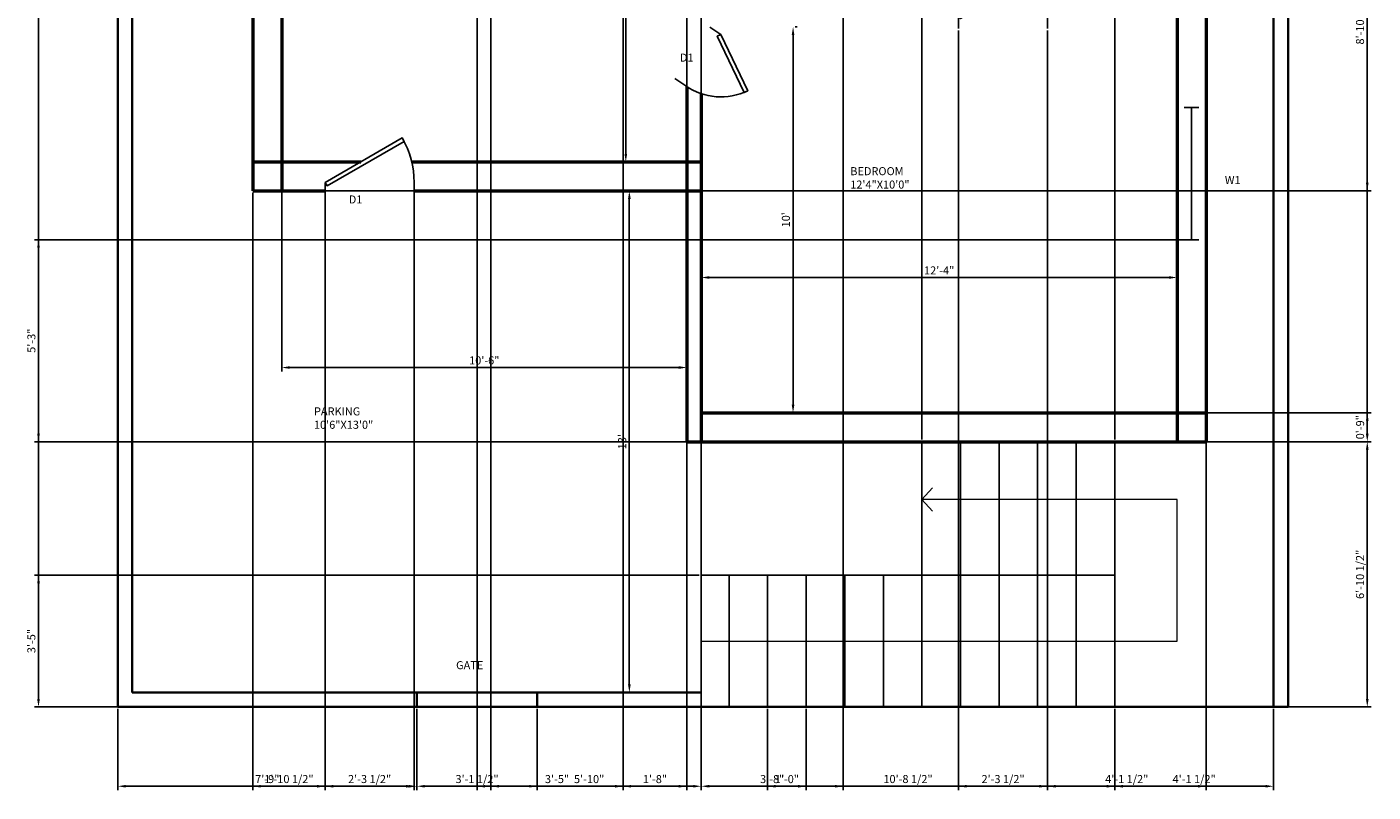
# Model space of a CAD drawing. Units: millimetres. Extents: x 2177 to 2598, y 1637 to 2185.
# Tile 1 of 2: x 2179 to 2598, y 1637 to 1875. Entities that reach past the tile are written whole.
import ezdxf

# ---------------------------------------------------------------- set-up
doc = ezdxf.new("R2010")
doc.units = ezdxf.units.MM
for name, color, linetype, lineweight in [('A-ANNO-DIMS', 150, 'Continuous', 18), ('A-ANNO-SYMB', 50, 'Continuous', 18), ('A-ANNO-TEXT', 40, 'Continuous', 18), ('A-AREA-IDEN', 40, 'Continuous', 25), ('A-WALL-SITE', 100, 'Continuous', 35), ('door', 130, 'Continuous', 25), ('steps', 50, 'Continuous', 25), ('walls', 100, 'Continuous', 50), ('windows', 10, 'Continuous', 25)]:
    doc.layers.add(name, color=color, linetype=linetype, lineweight=lineweight)
doc.styles.get("Standard").update_dxf_attribs({"font": 'arial.ttf'})
doc.dimstyles.new('ISO-25', dxfattribs={"dimtxt": 2.5, "dimasz": 2.5, "dimexe": 1.25, "dimexo": 0.625, "dimtad": 1, "dimlunit": 3, "dimtxsty": 'Standard', "dimcen": 2.5, "dimadec": 0, "dimazin": 0, "dimtfac": 1, "dimtmove": 0, "dimatfit": 3, "dimfxl": 1, "dimarcsym": 0})

# ---------------------------------------------------------------- blocks, each defined once
blk = doc.blocks.new('*U2')
for p, q in [((0, 0), (0, -6)), ((40, 0), (40, -6))]:
    blk.add_line(p, q)
blk.add_lwpolyline([(0, 0), (34.64, 20), (35.52, 18.48), (0.87, -1.52)], close=True)
blk.add_arc((0, 0), 40, 0, 30)
blk = doc.blocks.new('*U5')
for p, q in [((0, 0), (0, -6)), ((28, 0), (28, -6))]:
    blk.add_line(p, q)
blk.add_lwpolyline([(0, 0), (14, 24.25), (15.52, 23.37), (1.52, -0.88)], close=True)
blk.add_arc((0, 0), 28, 0, 60)
blk = doc.blocks.new('*U7')
for p, q in [((0, 4), (0, 0)), ((36, 4), (36, 0)), ((0, 2), (36, 2))]:
    blk.add_line(p, q)
blk = doc.blocks.new('*D15')
at = {"layer": 'A-ANNO-DIMS', "color": 0, "lineweight": -2, "transparency": 16777216}
for p, q in [((2344.56, 1989.02), (2366.75, 1989.02)), ((2365.5, 1835.52), (2365.5, 1986.52)), ((2344.56, 1833.02), (2366.75, 1833.02))]:
    blk.add_line(p, q, dxfattribs=at)
at = {"layer": 'A-ANNO-DIMS', "color": 0, "transparency": 16777216}
for points in [[(2365.08, 1986.52), (2365.91, 1986.52), (2365.5, 1989.02)], [(2365.08, 1835.52), (2365.91, 1835.52), (2365.5, 1833.02)]]:
    blk.add_solid(points, dxfattribs=at)
at = {"layer": 'Defpoints', "color": 0, "transparency": 16777216}
for p in [(2343.93, 1989.02), (2365.5, 1989.02), (2343.93, 1833.02)]:
    blk.add_point(p, dxfattribs=at)
at = {"layer": 'A-ANNO-DIMS', "color": 0, "transparency": 16777216, "insert": (2363.59, 1911.02), "char_height": 2.5, "attachment_point": 5, "rotation": 90}
blk.add_mtext("13'", dxfattribs=at)
blk = doc.blocks.new('*D16')
at = {"layer": 'A-ANNO-DIMS', "color": 0, "lineweight": -2, "transparency": 16777216}
for p, q in [((2344.93, 1824.02), (2367.84, 1824.02)), ((2366.59, 1821.52), (2366.59, 1670.52)), ((2344.93, 1668.02), (2367.84, 1668.02))]:
    blk.add_line(p, q, dxfattribs=at)
at = {"layer": 'A-ANNO-DIMS', "color": 0, "transparency": 16777216}
for points in [[(2366.18, 1821.52), (2367.01, 1821.52), (2366.59, 1824.02)], [(2366.18, 1670.52), (2367.01, 1670.52), (2366.59, 1668.02)]]:
    blk.add_solid(points, dxfattribs=at)
at = {"layer": 'Defpoints', "color": 0, "transparency": 16777216}
for p in [(2344.31, 1824.02), (2344.31, 1668.02), (2366.59, 1668.02)]:
    blk.add_point(p, dxfattribs=at)
at = {"layer": 'A-ANNO-DIMS', "color": 0, "transparency": 16777216, "insert": (2364.69, 1746.02), "char_height": 2.5, "attachment_point": 5, "rotation": 90}
blk.add_mtext("13'", dxfattribs=at)
blk = doc.blocks.new('*D17')
at = {"layer": 'A-ANNO-DIMS', "color": 0, "lineweight": -2, "transparency": 16777216}
for p, q in [((2258.47, 1832.4), (2258.47, 1767.82)), ((2384.47, 1832.4), (2384.47, 1767.82)), ((2260.97, 1769.07), (2381.97, 1769.07))]:
    blk.add_line(p, q, dxfattribs=at)
at = {"layer": 'A-ANNO-DIMS', "color": 0, "transparency": 16777216}
for points in [[(2260.97, 1769.49), (2260.97, 1768.66), (2258.47, 1769.07)], [(2381.97, 1769.49), (2381.97, 1768.66), (2384.47, 1769.07)]]:
    blk.add_solid(points, dxfattribs=at)
at = {"layer": 'Defpoints', "color": 0, "transparency": 16777216}
for p in [(2258.47, 1833.02), (2384.47, 1833.02), (2384.47, 1769.07)]:
    blk.add_point(p, dxfattribs=at)
at = {"layer": 'A-ANNO-DIMS', "color": 0, "transparency": 16777216, "insert": (2321.47, 1770.97), "char_height": 2.5, "attachment_point": 5}
blk.add_mtext('10\'-6"', dxfattribs=at)
blk = doc.blocks.new('*D18')
at = {"layer": 'A-ANNO-DIMS', "color": 0, "lineweight": -2, "transparency": 16777216}
for p, q in [((2417.52, 1757.52), (2417.52, 1872.52)), ((2418.14, 1875.02), (2418.77, 1875.02)), ((2418.14, 1755.02), (2418.77, 1755.02))]:
    blk.add_line(p, q, dxfattribs=at)
at = {"layer": 'A-ANNO-DIMS', "color": 0, "transparency": 16777216}
for points in [[(2417.1, 1872.52), (2417.93, 1872.52), (2417.52, 1875.02)], [(2417.1, 1757.52), (2417.93, 1757.52), (2417.52, 1755.02)]]:
    blk.add_solid(points, dxfattribs=at)
at = {"layer": 'Defpoints', "color": 0, "transparency": 16777216}
for p in [(2417.52, 1875.02), (2417.52, 1875.02), (2417.52, 1755.02)]:
    blk.add_point(p, dxfattribs=at)
at = {"layer": 'A-ANNO-DIMS', "color": 0, "transparency": 16777216, "insert": (2415.61, 1815.02), "char_height": 2.5, "attachment_point": 5, "rotation": 90}
blk.add_mtext("10'", dxfattribs=at)
blk = doc.blocks.new('*D19')
at = {"layer": 'A-ANNO-DIMS', "color": 0, "lineweight": -2, "transparency": 16777216}
for p, q in [((2388.97, 1812.3), (2388.97, 1795.82)), ((2536.97, 1812.3), (2536.97, 1795.82)), ((2391.47, 1797.07), (2534.47, 1797.07))]:
    blk.add_line(p, q, dxfattribs=at)
at = {"layer": 'A-ANNO-DIMS', "color": 0, "transparency": 16777216}
for points in [[(2391.47, 1797.49), (2391.47, 1796.66), (2388.97, 1797.07)], [(2534.47, 1797.49), (2534.47, 1796.66), (2536.97, 1797.07)]]:
    blk.add_solid(points, dxfattribs=at)
at = {"layer": 'Defpoints', "color": 0, "transparency": 16777216}
for p in [(2388.97, 1812.93), (2536.97, 1812.93), (2536.97, 1797.07)]:
    blk.add_point(p, dxfattribs=at)
at = {"layer": 'A-ANNO-DIMS', "color": 0, "transparency": 16777216, "insert": (2462.97, 1798.95), "char_height": 2.5, "attachment_point": 5}
blk.add_mtext('12\'-4"', dxfattribs=at)
blk = doc.blocks.new('*D25')
at = {"layer": 'A-ANNO-DIMS', "color": 0, "lineweight": -2, "transparency": 16777216}
for p, q in [((2206.84, 2154.52), (2181.57, 2154.52)), ((2182.82, 1666.02), (2182.82, 2152.02)), ((2206.84, 1663.52), (2181.57, 1663.52))]:
    blk.add_line(p, q, dxfattribs=at)
at = {"layer": 'A-ANNO-DIMS', "color": 0, "transparency": 16777216}
for points in [[(2182.4, 2152.02), (2183.24, 2152.02), (2182.82, 2154.52)], [(2182.4, 1666.02), (2183.24, 1666.02), (2182.82, 1663.52)]]:
    blk.add_solid(points, dxfattribs=at)
at = {"layer": 'Defpoints', "color": 0, "transparency": 16777216}
for p in [(2182.82, 2154.52), (2207.47, 2154.52), (2207.47, 1663.52)]:
    blk.add_point(p, dxfattribs=at)
at = {"layer": 'A-ANNO-DIMS', "color": 0, "transparency": 16777216, "insert": (2180.92, 1909.02), "char_height": 2.5, "attachment_point": 5, "rotation": 90}
blk.add_mtext('40\'-11"', dxfattribs=at)
blk = doc.blocks.new('*D27')
at = {"layer": 'A-ANNO-DIMS', "color": 0, "lineweight": -2, "transparency": 16777216}
for p, q in [((2546.59, 2122.52), (2597.37, 2122.52)), ((2596.12, 2120.02), (2596.12, 1748.52)), ((2546.59, 1746.02), (2597.37, 1746.02))]:
    blk.add_line(p, q, dxfattribs=at)
at = {"layer": 'A-ANNO-DIMS', "color": 0, "transparency": 16777216}
for points in [[(2595.7, 2120.02), (2596.54, 2120.02), (2596.12, 2122.52)], [(2595.7, 1748.52), (2596.54, 1748.52), (2596.12, 1746.02)]]:
    blk.add_solid(points, dxfattribs=at)
at = {"layer": 'Defpoints', "color": 0, "transparency": 16777216}
for p in [(2545.97, 2122.52), (2545.97, 1746.02), (2596.12, 1746.02)]:
    blk.add_point(p, dxfattribs=at)
at = {"layer": 'A-ANNO-DIMS', "color": 0, "transparency": 16777216, "insert": (2594.2, 1934.27), "char_height": 2.5, "attachment_point": 5, "rotation": 90}
blk.add_mtext('31\'-4 1/2"', dxfattribs=at)
blk = doc.blocks.new('*D28')
at = {"layer": 'A-ANNO-DIMS', "color": 0, "lineweight": -2, "transparency": 16777216}
for p, q in [((2546.59, 1755.02), (2597.37, 1755.02)), ((2596.12, 1752.52), (2596.12, 1748.52)), ((2546.59, 1746.02), (2597.37, 1746.02))]:
    blk.add_line(p, q, dxfattribs=at)
at = {"layer": 'A-ANNO-DIMS', "color": 0, "transparency": 16777216}
for points in [[(2595.7, 1752.52), (2596.54, 1752.52), (2596.12, 1755.02)], [(2595.7, 1748.52), (2596.54, 1748.52), (2596.12, 1746.02)]]:
    blk.add_solid(points, dxfattribs=at)
at = {"layer": 'Defpoints', "color": 0, "transparency": 16777216}
for p in [(2545.97, 1755.02), (2545.97, 1746.02), (2596.12, 1746.02)]:
    blk.add_point(p, dxfattribs=at)
at = {"layer": 'A-ANNO-DIMS', "color": 0, "transparency": 16777216, "insert": (2594.22, 1750.52), "char_height": 2.5, "attachment_point": 5, "rotation": 90}
blk.add_mtext('0\'-9"', dxfattribs=at)
blk = doc.blocks.new('*D30')
at = {"layer": 'A-ANNO-DIMS', "color": 0, "lineweight": -2, "transparency": 16777216}
for p, q in [((2300.47, 1662.9), (2300.47, 1637.62)), ((2337.97, 1662.9), (2337.97, 1637.62)), ((2302.97, 1638.87), (2335.47, 1638.87))]:
    blk.add_line(p, q, dxfattribs=at)
at = {"layer": 'A-ANNO-DIMS', "color": 0, "transparency": 16777216}
for points in [[(2302.97, 1639.29), (2302.97, 1638.46), (2300.47, 1638.87)], [(2335.47, 1639.29), (2335.47, 1638.46), (2337.97, 1638.87)]]:
    blk.add_solid(points, dxfattribs=at)
at = {"layer": 'Defpoints', "color": 0, "transparency": 16777216}
for p in [(2300.47, 1663.52), (2337.97, 1663.52), (2337.97, 1638.87)]:
    blk.add_point(p, dxfattribs=at)
at = {"layer": 'A-ANNO-DIMS', "color": 0, "transparency": 16777216, "insert": (2319.22, 1640.79), "char_height": 2.5, "attachment_point": 5}
blk.add_mtext('3\'-1 1/2"', dxfattribs=at)
blk = doc.blocks.new('*D31')
at = {"layer": 'A-ANNO-DIMS', "color": 0, "lineweight": -2, "transparency": 16777216}
for p, q in [((2207.47, 1662.9), (2207.47, 1637.62)), ((2300.47, 1662.9), (2300.47, 1637.62)), ((2209.97, 1638.87), (2297.97, 1638.87))]:
    blk.add_line(p, q, dxfattribs=at)
at = {"layer": 'A-ANNO-DIMS', "color": 0, "transparency": 16777216}
for points in [[(2209.97, 1639.29), (2209.97, 1638.46), (2207.47, 1638.87)], [(2297.97, 1639.29), (2297.97, 1638.46), (2300.47, 1638.87)]]:
    blk.add_solid(points, dxfattribs=at)
at = {"layer": 'Defpoints', "color": 0, "transparency": 16777216}
for p in [(2207.47, 1663.52), (2300.47, 1663.52), (2300.47, 1638.87)]:
    blk.add_point(p, dxfattribs=at)
at = {"layer": 'A-ANNO-DIMS', "color": 0, "transparency": 16777216, "insert": (2253.97, 1640.77), "char_height": 2.5, "attachment_point": 5}
blk.add_mtext('7\'-9"', dxfattribs=at)
blk = doc.blocks.new('*D32')
at = {"layer": 'A-ANNO-DIMS', "color": 0, "lineweight": -2, "transparency": 16777216}
for p, q in [((2271.98, 1823.4), (2271.98, 1637.62)), ((2299.64, 1823.4), (2299.64, 1637.62)), ((2274.48, 1638.87), (2297.14, 1638.87))]:
    blk.add_line(p, q, dxfattribs=at)
at = {"layer": 'A-ANNO-DIMS', "color": 0, "transparency": 16777216}
for points in [[(2274.48, 1639.29), (2274.48, 1638.46), (2271.98, 1638.87)], [(2297.14, 1639.29), (2297.14, 1638.46), (2299.64, 1638.87)]]:
    blk.add_solid(points, dxfattribs=at)
at = {"layer": 'Defpoints', "color": 0, "transparency": 16777216}
for p in [(2271.98, 1824.02), (2299.64, 1824.02), (2299.64, 1638.87)]:
    blk.add_point(p, dxfattribs=at)
at = {"layer": 'A-ANNO-DIMS', "color": 0, "transparency": 16777216, "insert": (2285.81, 1640.79), "char_height": 2.5, "attachment_point": 5}
blk.add_mtext('2\'-3 1/2"', dxfattribs=at)
blk = doc.blocks.new('*D33')
at = {"layer": 'A-ANNO-DIMS', "color": 0, "lineweight": -2, "transparency": 16777216}
for p, q in [((2323.55, 2116.57), (2323.55, 1637.62)), ((2364.65, 2116.57), (2364.65, 1637.62)), ((2326.05, 1638.87), (2362.15, 1638.87))]:
    blk.add_line(p, q, dxfattribs=at)
at = {"layer": 'A-ANNO-DIMS', "color": 0, "transparency": 16777216}
for points in [[(2326.05, 1639.29), (2326.05, 1638.46), (2323.55, 1638.87)], [(2362.15, 1639.29), (2362.15, 1638.46), (2364.65, 1638.87)]]:
    blk.add_solid(points, dxfattribs=at)
at = {"layer": 'Defpoints', "color": 0, "transparency": 16777216}
for p in [(2323.55, 2117.19), (2364.65, 2117.19), (2364.65, 1638.87)]:
    blk.add_point(p, dxfattribs=at)
at = {"layer": 'A-ANNO-DIMS', "color": 0, "transparency": 16777216, "insert": (2344.1, 1640.78), "char_height": 2.5, "attachment_point": 5}
blk.add_mtext('3\'-5"', dxfattribs=at)
blk = doc.blocks.new('*D35')
at = {"layer": 'A-ANNO-DIMS', "color": 0, "lineweight": -2, "transparency": 16777216}
for p, q in [((2457.6, 1746.65), (2457.6, 2180.42)), ((2460.1, 2179.17), (2515.1, 2179.17)), ((2517.6, 1746.65), (2517.6, 2180.42))]:
    blk.add_line(p, q, dxfattribs=at)
at = {"layer": 'A-ANNO-DIMS', "color": 0, "transparency": 16777216}
for points in [[(2460.1, 2179.59), (2460.1, 2178.76), (2457.6, 2179.17)], [(2515.1, 2179.59), (2515.1, 2178.76), (2517.6, 2179.17)]]:
    blk.add_solid(points, dxfattribs=at)
at = {"layer": 'Defpoints', "color": 0, "transparency": 16777216}
for p in [(2517.6, 2179.17), (2457.6, 1746.02), (2517.6, 1746.02)]:
    blk.add_point(p, dxfattribs=at)
at = {"layer": 'A-ANNO-DIMS', "color": 0, "transparency": 16777216, "insert": (2487.6, 2181.07), "char_height": 2.5, "attachment_point": 5}
blk.add_mtext('5\'-0"', dxfattribs=at)
blk = doc.blocks.new('*D36')
at = {"layer": 'A-ANNO-DIMS', "color": 0, "lineweight": -2, "transparency": 16777216}
for p, q in [((2409.6, 1662.9), (2409.6, 1637.62)), ((2421.6, 1662.9), (2421.6, 1637.62)), ((2412.1, 1638.87), (2419.1, 1638.87))]:
    blk.add_line(p, q, dxfattribs=at)
at = {"layer": 'A-ANNO-DIMS', "color": 0, "transparency": 16777216}
for points in [[(2412.1, 1639.29), (2412.1, 1638.46), (2409.6, 1638.87)], [(2419.1, 1639.29), (2419.1, 1638.46), (2421.6, 1638.87)]]:
    blk.add_solid(points, dxfattribs=at)
at = {"layer": 'Defpoints', "color": 0, "transparency": 16777216}
for p in [(2409.6, 1663.52), (2421.6, 1663.52), (2421.6, 1638.87)]:
    blk.add_point(p, dxfattribs=at)
at = {"layer": 'A-ANNO-DIMS', "color": 0, "transparency": 16777216, "insert": (2415.6, 1640.77), "char_height": 2.5, "attachment_point": 5}
blk.add_mtext('1\'-0"', dxfattribs=at)
blk = doc.blocks.new('*D37')
at = {"layer": 'A-ANNO-DIMS', "color": 0, "lineweight": -2, "transparency": 16777216}
for p, q in [((2388.34, 1704.52), (2181.57, 1704.52)), ((2182.82, 1666.02), (2182.82, 1702.02)), ((2388.34, 1663.52), (2181.57, 1663.52))]:
    blk.add_line(p, q, dxfattribs=at)
at = {"layer": 'A-ANNO-DIMS', "color": 0, "transparency": 16777216}
for points in [[(2182.4, 1702.02), (2183.24, 1702.02), (2182.82, 1704.52)], [(2182.4, 1666.02), (2183.24, 1666.02), (2182.82, 1663.52)]]:
    blk.add_solid(points, dxfattribs=at)
at = {"layer": 'Defpoints', "color": 0, "transparency": 16777216}
for p in [(2182.82, 1704.52), (2388.97, 1704.52), (2388.97, 1663.52)]:
    blk.add_point(p, dxfattribs=at)
at = {"layer": 'A-ANNO-DIMS', "color": 0, "transparency": 16777216, "insert": (2180.92, 1684.02), "char_height": 2.5, "attachment_point": 5, "rotation": 90}
blk.add_mtext('3\'-5"', dxfattribs=at)
blk = doc.blocks.new('*D38')
at = {"layer": 'A-ANNO-DIMS', "color": 0, "lineweight": -2, "transparency": 16777216}
for p, q in [((2388.97, 1662.9), (2388.97, 1637.62)), ((2517.6, 1662.9), (2517.6, 1637.62)), ((2391.47, 1638.87), (2515.1, 1638.87))]:
    blk.add_line(p, q, dxfattribs=at)
at = {"layer": 'A-ANNO-DIMS', "color": 0, "transparency": 16777216}
for points in [[(2391.47, 1639.29), (2391.47, 1638.46), (2388.97, 1638.87)], [(2515.1, 1639.29), (2515.1, 1638.46), (2517.6, 1638.87)]]:
    blk.add_solid(points, dxfattribs=at)
at = {"layer": 'Defpoints', "color": 0, "transparency": 16777216}
for p in [(2388.97, 1663.52), (2517.6, 1663.52), (2517.6, 1638.87)]:
    blk.add_point(p, dxfattribs=at)
at = {"layer": 'A-ANNO-DIMS', "color": 0, "transparency": 16777216, "insert": (2453.28, 1640.79), "char_height": 2.5, "attachment_point": 5}
blk.add_mtext('10\'-8 1/2"', dxfattribs=at)
blk = doc.blocks.new('*D39')
at = {"layer": 'A-ANNO-DIMS', "color": 0, "lineweight": -2, "transparency": 16777216}
for p, q in [((2517.6, 1662.9), (2517.6, 1637.62)), ((2566.97, 1662.9), (2566.97, 1637.62)), ((2520.1, 1638.87), (2564.47, 1638.87))]:
    blk.add_line(p, q, dxfattribs=at)
at = {"layer": 'A-ANNO-DIMS', "color": 0, "transparency": 16777216}
for points in [[(2520.1, 1639.29), (2520.1, 1638.46), (2517.6, 1638.87)], [(2564.47, 1639.29), (2564.47, 1638.46), (2566.97, 1638.87)]]:
    blk.add_solid(points, dxfattribs=at)
at = {"layer": 'Defpoints', "color": 0, "transparency": 16777216}
for p in [(2517.6, 1663.52), (2566.97, 1663.52), (2566.97, 1638.87)]:
    blk.add_point(p, dxfattribs=at)
at = {"layer": 'A-ANNO-DIMS', "color": 0, "transparency": 16777216, "insert": (2542.28, 1640.79), "char_height": 2.5, "attachment_point": 5}
blk.add_mtext('4\'-1 1/2"', dxfattribs=at)
blk = doc.blocks.new('*D40')
at = {"layer": 'A-ANNO-DIMS', "color": 0, "lineweight": -2, "transparency": 16777216}
for p, q in [((2469.01, 1873.88), (2469.01, 1637.62)), ((2496.67, 1873.88), (2496.67, 1637.62)), ((2471.51, 1638.87), (2494.17, 1638.87))]:
    blk.add_line(p, q, dxfattribs=at)
at = {"layer": 'A-ANNO-DIMS', "color": 0, "transparency": 16777216}
for points in [[(2471.51, 1639.29), (2471.51, 1638.46), (2469.01, 1638.87)], [(2494.17, 1639.29), (2494.17, 1638.46), (2496.67, 1638.87)]]:
    blk.add_solid(points, dxfattribs=at)
at = {"layer": 'Defpoints', "color": 0, "transparency": 16777216}
for p in [(2469.01, 1874.51), (2496.67, 1874.51), (2496.67, 1638.87)]:
    blk.add_point(p, dxfattribs=at)
at = {"layer": 'A-ANNO-DIMS', "color": 0, "transparency": 16777216, "insert": (2482.84, 1640.79), "char_height": 2.5, "attachment_point": 5}
blk.add_mtext('2\'-3 1/2"', dxfattribs=at)
blk = doc.blocks.new('*D41')
at = {"layer": 'A-ANNO-DIMS', "color": 0, "lineweight": -2, "transparency": 16777216}
for p, q in [((2249.47, 1823.4), (2249.47, 1637.62)), ((2271.98, 1823.4), (2271.98, 1637.62)), ((2251.97, 1638.87), (2269.48, 1638.87))]:
    blk.add_line(p, q, dxfattribs=at)
at = {"layer": 'A-ANNO-DIMS', "color": 0, "transparency": 16777216}
for points in [[(2251.97, 1639.29), (2251.97, 1638.46), (2249.47, 1638.87)], [(2269.48, 1639.29), (2269.48, 1638.46), (2271.98, 1638.87)]]:
    blk.add_solid(points, dxfattribs=at)
at = {"layer": 'Defpoints', "color": 0, "transparency": 16777216}
for p in [(2249.47, 1824.02), (2271.98, 1824.02), (2271.98, 1638.87)]:
    blk.add_point(p, dxfattribs=at)
at = {"layer": 'A-ANNO-DIMS', "color": 0, "transparency": 16777216, "insert": (2260.72, 1640.79), "char_height": 2.5, "attachment_point": 5}
blk.add_mtext('1\'-10 1/2"', dxfattribs=at)
blk = doc.blocks.new('*D43')
at = {"layer": 'A-ANNO-DIMS', "color": 0, "lineweight": -2, "transparency": 16777216}
for p, q in [((2545.97, 1878.9), (2545.97, 1637.62)), ((2496.67, 1873.88), (2496.67, 1637.62)), ((2499.17, 1638.87), (2543.47, 1638.87))]:
    blk.add_line(p, q, dxfattribs=at)
at = {"layer": 'A-ANNO-DIMS', "color": 0, "transparency": 16777216}
for points in [[(2499.17, 1639.29), (2499.17, 1638.46), (2496.67, 1638.87)], [(2543.47, 1639.29), (2543.47, 1638.46), (2545.97, 1638.87)]]:
    blk.add_solid(points, dxfattribs=at)
at = {"layer": 'Defpoints', "color": 0, "transparency": 16777216}
for p in [(2545.97, 1879.52), (2496.67, 1874.51), (2545.97, 1638.87)]:
    blk.add_point(p, dxfattribs=at)
at = {"layer": 'A-ANNO-DIMS', "color": 0, "transparency": 16777216, "insert": (2521.32, 1640.79), "char_height": 2.5, "attachment_point": 5}
blk.add_mtext('4\'-1 1/2"', dxfattribs=at)
blk = doc.blocks.new('*D45')
at = {"layer": 'A-ANNO-DIMS', "color": 0, "lineweight": -2, "transparency": 16777216}
for p, q in [((2518.22, 1746.02), (2597.37, 1746.02)), ((2596.12, 1666.02), (2596.12, 1743.52)), ((2518.22, 1663.52), (2597.37, 1663.52))]:
    blk.add_line(p, q, dxfattribs=at)
at = {"layer": 'A-ANNO-DIMS', "color": 0, "transparency": 16777216}
for points in [[(2595.7, 1743.52), (2596.54, 1743.52), (2596.12, 1746.02)], [(2595.7, 1666.02), (2596.54, 1666.02), (2596.12, 1663.52)]]:
    blk.add_solid(points, dxfattribs=at)
at = {"layer": 'Defpoints', "color": 0, "transparency": 16777216}
for p in [(2517.6, 1746.02), (2596.12, 1746.02), (2517.6, 1663.52)]:
    blk.add_point(p, dxfattribs=at)
at = {"layer": 'A-ANNO-DIMS', "color": 0, "transparency": 16777216, "insert": (2594.2, 1704.77), "char_height": 2.5, "attachment_point": 5, "rotation": 90}
blk.add_mtext('6\'-10 1/2"', dxfattribs=at)
blk = doc.blocks.new('*D47')
at = {"layer": 'A-ANNO-DIMS', "color": 0, "lineweight": -2, "transparency": 16777216}
for p, q in [((2319.22, 1988.4), (2319.22, 1637.62)), ((2388.97, 1988.4), (2388.97, 1637.62)), ((2321.72, 1638.87), (2386.47, 1638.87))]:
    blk.add_line(p, q, dxfattribs=at)
at = {"layer": 'A-ANNO-DIMS', "color": 0, "transparency": 16777216}
for points in [[(2321.72, 1639.29), (2321.72, 1638.46), (2319.22, 1638.87)], [(2386.47, 1639.29), (2386.47, 1638.46), (2388.97, 1638.87)]]:
    blk.add_solid(points, dxfattribs=at)
at = {"layer": 'Defpoints', "color": 0, "transparency": 16777216}
for p in [(2319.22, 1989.02), (2388.97, 1989.02), (2388.97, 1638.87)]:
    blk.add_point(p, dxfattribs=at)
at = {"layer": 'A-ANNO-DIMS', "color": 0, "transparency": 16777216, "insert": (2354.09, 1640.77), "char_height": 2.5, "attachment_point": 5}
blk.add_mtext('5\'-10"', dxfattribs=at)
blk = doc.blocks.new('*D48')
at = {"layer": 'A-ANNO-DIMS', "color": 0, "lineweight": -2, "transparency": 16777216}
for p, q in [((2388.97, 2121.9), (2388.97, 1637.62)), ((2433.07, 2116.49), (2433.07, 1637.62)), ((2391.47, 1638.87), (2430.57, 1638.87))]:
    blk.add_line(p, q, dxfattribs=at)
at = {"layer": 'A-ANNO-DIMS', "color": 0, "transparency": 16777216}
for points in [[(2391.47, 1639.29), (2391.47, 1638.46), (2388.97, 1638.87)], [(2430.57, 1639.29), (2430.57, 1638.46), (2433.07, 1638.87)]]:
    blk.add_solid(points, dxfattribs=at)
at = {"layer": 'Defpoints', "color": 0, "transparency": 16777216}
for p in [(2388.97, 2122.52), (2433.07, 2117.11), (2433.07, 1638.87)]:
    blk.add_point(p, dxfattribs=at)
at = {"layer": 'A-ANNO-DIMS', "color": 0, "transparency": 16777216, "insert": (2411.02, 1640.78), "char_height": 2.5, "attachment_point": 5}
blk.add_mtext('3\'-8"', dxfattribs=at)
blk = doc.blocks.new('*D50')
at = {"layer": 'A-ANNO-DIMS', "color": 0, "lineweight": -2, "transparency": 16777216}
for p, q in [((2254.73, 1930.31), (2597.37, 1930.31)), ((2596.12, 1826.52), (2596.12, 1927.81)), ((2259.09, 1824.02), (2597.37, 1824.02))]:
    blk.add_line(p, q, dxfattribs=at)
at = {"layer": 'A-ANNO-DIMS', "color": 0, "transparency": 16777216}
for points in [[(2595.7, 1927.81), (2596.54, 1927.81), (2596.12, 1930.31)], [(2595.7, 1826.52), (2596.54, 1826.52), (2596.12, 1824.02)]]:
    blk.add_solid(points, dxfattribs=at)
at = {"layer": 'Defpoints', "color": 0, "transparency": 16777216}
for p in [(2254.11, 1930.31), (2596.12, 1930.31), (2258.47, 1824.02)]:
    blk.add_point(p, dxfattribs=at)
at = {"layer": 'A-ANNO-DIMS', "color": 0, "transparency": 16777216, "insert": (2594.2, 1877.17), "char_height": 2.5, "attachment_point": 5, "rotation": 90}
blk.add_mtext('8\'-10 1/2"', dxfattribs=at)
blk = doc.blocks.new('*D52')
at = {"layer": 'A-ANNO-DIMS', "color": 0, "lineweight": -2, "transparency": 16777216}
for p, q in [((2540.85, 1808.81), (2181.57, 1808.81)), ((2182.82, 1806.31), (2182.82, 1748.52)), ((2536.34, 1746.02), (2181.57, 1746.02))]:
    blk.add_line(p, q, dxfattribs=at)
at = {"layer": 'A-ANNO-DIMS', "color": 0, "transparency": 16777216}
for points in [[(2182.4, 1806.31), (2183.24, 1806.31), (2182.82, 1808.81)], [(2182.4, 1748.52), (2183.24, 1748.52), (2182.82, 1746.02)]]:
    blk.add_solid(points, dxfattribs=at)
at = {"layer": 'Defpoints', "color": 0, "transparency": 16777216}
for p in [(2541.47, 1808.81), (2182.82, 1746.02), (2536.97, 1746.02)]:
    blk.add_point(p, dxfattribs=at)
at = {"layer": 'A-ANNO-DIMS', "color": 0, "transparency": 16777216, "insert": (2180.92, 1777.42), "char_height": 2.5, "attachment_point": 5, "rotation": 90}
blk.add_mtext('5\'-3"', dxfattribs=at)
blk = doc.blocks.new('*D53')
at = {"layer": 'A-ANNO-DIMS', "color": 0, "lineweight": -2, "transparency": 16777216}
for p, q in [((2384.47, 2121.9), (2384.47, 1637.62)), ((2364.65, 2116.57), (2364.65, 1637.62)), ((2367.15, 1638.87), (2381.97, 1638.87))]:
    blk.add_line(p, q, dxfattribs=at)
at = {"layer": 'A-ANNO-DIMS', "color": 0, "transparency": 16777216}
for points in [[(2367.15, 1639.29), (2367.15, 1638.46), (2364.65, 1638.87)], [(2381.97, 1639.29), (2381.97, 1638.46), (2384.47, 1638.87)]]:
    blk.add_solid(points, dxfattribs=at)
at = {"layer": 'Defpoints', "color": 0, "transparency": 16777216}
for p in [(2384.47, 2122.52), (2364.65, 2117.19), (2384.47, 1638.87)]:
    blk.add_point(p, dxfattribs=at)
at = {"layer": 'A-ANNO-DIMS', "color": 0, "transparency": 16777216, "insert": (2374.56, 1640.77), "char_height": 2.5, "attachment_point": 5}
blk.add_mtext('1\'-8"', dxfattribs=at)

msp = doc.modelspace()

# ---------------------------------------------------------------- linework, layer by layer
at = {"layer": 'A-ANNO-SYMB'}
for p, q in [((2457.598, 1728.042), (2460.872, 1731.701)), ((2536.97, 1728.042), (2457.598, 1728.042)), ((2457.598, 1728.042), (2457.598, 1728.042)), ((2457.598, 1728.042), (2460.872, 1724.383)), ((2536.97, 1684.023), (2536.97, 1728.042)), ((2388.97, 1684.023), (2536.97, 1684.023))]:
    msp.add_line(p, q, dxfattribs=at)
at = {"layer": 'A-WALL-SITE'}
for p, q in [((2207.47, 2154.523), (2207.47, 1663.523)), ((2211.97, 2154.523), (2211.97, 1668.023)), ((2566.97, 1663.523), (2566.97, 2154.523)), ((2571.47, 1663.523), (2571.47, 2154.523)), ((2211.97, 1668.023), (2388.97, 1668.023)), ((2300.47, 1668.023), (2300.47, 1663.523)), ((2300.47, 1663.523), (2300.47, 1668.023)), ((2300.47, 1668.023), (2300.47, 1668.023)), ((2337.97, 1668.023), (2337.97, 1663.523)), ((2207.47, 1663.523), (2505.598, 1663.523)), ((2505.598, 1663.523), (2571.47, 1663.523))]:
    msp.add_line(p, q, dxfattribs=at)
at = {"layer": 'steps'}
for p, q in [((2388.97, 1746.023), (2388.97, 1663.523)), ((2388.97, 1746.023), (2388.97, 1705.023)), ((2457.598, 1746.023), (2457.598, 1663.523)), ((2469.598, 1746.023), (2469.598, 1663.523)), ((2481.598, 1746.023), (2481.598, 1663.523)), ((2493.598, 1746.023), (2493.598, 1663.523)), ((2505.598, 1746.023), (2505.598, 1663.523)), ((2517.598, 1704.523), (2517.598, 1746.023)), ((2517.598, 1746.023), (2517.598, 1663.523)), ((2388.97, 1663.523), (2388.97, 1704.523)), ((2388.97, 1663.523), (2388.97, 1704.523)), ((2388.97, 1704.523), (2517.598, 1704.523)), ((2397.598, 1704.523), (2397.598, 1663.523)), ((2409.598, 1704.523), (2409.598, 1663.523)), ((2421.598, 1704.523), (2421.598, 1663.523)), ((2433.598, 1704.523), (2433.598, 1663.523)), ((2445.598, 1704.523), (2445.598, 1663.523)), ((2388.97, 1663.523), (2388.97, 1699.523))]:
    msp.add_line(p, q, dxfattribs=at)
at = {"layer": 'walls'}
for p, q in [((2536.97, 2122.523), (2536.97, 1746.023)), ((2545.97, 2122.523), (2545.97, 1746.023)), ((2258.47, 2068.811), (2258.47, 1824.023)), ((2249.47, 2068.167), (2249.47, 1824.023)), ((2384.47, 1856.396), (2384.47, 1824.023)), ((2384.47, 1854.228), (2384.47, 1746.023)), ((2388.97, 1854.228), (2388.97, 1746.023)), ((2249.47, 1833.023), (2283.05, 1833.023)), ((2298.896, 1833.023), (2388.97, 1833.023)), ((2249.47, 1824.023), (2271.978, 1824.023)), ((2299.644, 1824.023), (2388.97, 1824.023)), ((2388.97, 1755.023), (2545.97, 1755.023)), ((2384.47, 1746.023), (2545.97, 1746.023))]:
    msp.add_line(p, q, dxfattribs=at)

# ---------------------------------------------------------------- block references
at = {"layer": 'door', "xscale": 0.6916711511996688, "yscale": 0.6916711511996688, "zscale": 0.6916711511996688}
for p in [(2469.006, 1878.656), (2271.978, 1826.63)]:
    msp.add_blockref('*U2', p, dxfattribs=at)
at = {"layer": 'door', "xscale": 0.6916711511996688, "yscale": 0.6916711511996688, "zscale": 0.6916711511996688, "rotation": 235.6478842644134}
msp.add_blockref('*U5', (2395.055, 1872.614), dxfattribs=at)
at = {"layer": 'windows', "xscale": 1.141567510768898, "yscale": 1.141567510768898, "zscale": 1.141567510768898, "rotation": 90}
msp.add_blockref('*U7', (2543.757, 1808.811), dxfattribs=at)

# ---------------------------------------------------------------- texts
at = {"layer": 'A-ANNO-TEXT', "char_height": 2.5, "attachment_point": 1}
for s, width, insert in [('D1', 10.28271, (2382.317, 1866.693)), ('W1', 9.9642, (2551.829, 1828.601)), ('D1', 13.6379, (2279.317, 1822.592)), ('GATE', 53.55165, (2312.704, 1677.772))]:
    msp.add_mtext_dynamic_manual_height_columns(s, width=width, gutter_width=12.5, heights=[0], dxfattribs=dict(at, insert=insert))
at = {"layer": 'A-AREA-IDEN', "char_height": 2.5, "attachment_point": 1}
for s, width, insert in [('BEDROOM\\P12\'4"X10\'0"', 56.06434, (2435.304, 1831.388)), ('PARKING\\P10\'6"X13\'0"', 77.52097, (2268.495, 1756.691))]:
    msp.add_mtext_dynamic_manual_height_columns(s, width=width, gutter_width=12.5, heights=[0], dxfattribs=dict(at, insert=insert))

# ---------------------------------------------------------------- dimensions: what is measured, and where the dimension line sits
at = {"layer": 'A-ANNO-DIMS'}
for base, p1, p2, override, picture, middle in [((2517.598, 2179.173), (2457.598, 1746.023), (2517.598, 1746.023), {"dimdec": 1, "dimlfac": 1, "dimrnd": 0, "dimzin": 1, "dimdsep": 46, "dimlunit": 4, "dimfrac": 2}, '*D35', (2487.598, 2181.074)), ((2384.47, 1638.873), (2364.645, 2117.193), (2384.47, 2122.523), {"dimdec": 1, "dimlfac": 1, "dimrnd": 0, "dimzin": 1, "dimdsep": 46, "dimlunit": 4, "dimfrac": 2}, '*D53', (2374.558, 1640.774)), ((2433.071, 1638.873), (2388.97, 2122.523), (2433.071, 2117.114), {"dimdec": 1, "dimlfac": 1, "dimrnd": 0, "dimzin": 1, "dimdsep": 46, "dimlunit": 4, "dimfrac": 2}, '*D48', (2411.02, 1640.775)), ((2364.645, 1638.873), (2323.549, 2117.193), (2364.645, 2117.193), {"dimdec": 1, "dimlfac": 1, "dimrnd": 0, "dimzin": 1, "dimdsep": 46, "dimlunit": 4, "dimfrac": 2}, '*D33', (2344.097, 1640.775)), ((2388.969775, 1638.87304), (2319.219775, 1989.02304), (2388.969775, 1989.02304), {"dimdec": 1, "dimlfac": 1, "dimrnd": 0, "dimzin": 1, "dimdsep": 46, "dimlunit": 4, "dimfrac": 2}, '*D47', (2354.094775, 1640.774472469)), ((2545.97, 1638.873), (2496.673, 1874.506), (2545.97, 1879.523), {"dimdec": 1, "dimlfac": 1, "dimrnd": 0, "dimzin": 1, "dimdsep": 46, "dimlunit": 4, "dimfrac": 2}, '*D43', (2521.322, 1640.791)), ((2496.673, 1638.873), (2469.006, 1874.506), (2496.673, 1874.506), {"dimdec": 1, "dimlfac": 1, "dimrnd": 0, "dimzin": 1, "dimdsep": 46, "dimlunit": 4, "dimfrac": 2}, '*D40', (2482.84, 1640.792)), ((2384.47, 1769.072), (2258.47, 1833.023), (2384.47, 1833.023), {"dimclrd": 0, "dimclre": 0, "dimclrt": 0}, '*D17', (2321.47, 1770.974)), ((2271.978, 1638.873), (2249.47, 1824.023), (2271.978, 1824.023), {"dimdec": 1, "dimlfac": 1, "dimrnd": 0, "dimzin": 1, "dimdsep": 46, "dimlunit": 4, "dimfrac": 2}, '*D41', (2260.724, 1640.791)), ((2299.644, 1638.873), (2271.978, 1824.023), (2299.644, 1824.023), {"dimdec": 1, "dimlfac": 1, "dimrnd": 0, "dimzin": 1, "dimdsep": 46, "dimlunit": 4, "dimfrac": 2}, '*D32', (2285.811, 1640.792)), ((2536.97, 1797.073), (2388.97, 1812.927), (2536.97, 1812.927), {"dimclrd": 0, "dimclre": 0, "dimclrt": 0}, '*D19', (2462.97, 1798.953)), ((2300.47, 1638.873), (2207.47, 1663.523), (2300.47, 1663.523), {"dimdec": 1, "dimlfac": 1, "dimrnd": 0, "dimzin": 1, "dimdsep": 46, "dimlunit": 4, "dimfrac": 2}, '*D31', (2253.97, 1640.774)), ((2337.97, 1638.873), (2300.47, 1663.523), (2337.97, 1663.523), {"dimdec": 1, "dimlfac": 1, "dimrnd": 0, "dimzin": 1, "dimdsep": 46, "dimlunit": 4, "dimfrac": 2}, '*D30', (2319.22, 1640.792)), ((2517.598, 1638.873), (2388.97, 1663.523), (2517.598, 1663.523), {"dimdec": 1, "dimlfac": 1, "dimrnd": 0, "dimzin": 1, "dimdsep": 46, "dimlunit": 4, "dimfrac": 2}, '*D38', (2453.284, 1640.791)), ((2421.598, 1638.873), (2409.598, 1663.523), (2421.598, 1663.523), {"dimdec": 1, "dimlfac": 1, "dimrnd": 0, "dimzin": 1, "dimdsep": 46, "dimlunit": 4, "dimfrac": 2}, '*D36', (2415.598, 1640.774)), ((2566.97, 1638.873), (2517.598, 1663.523), (2566.97, 1663.523), {"dimdec": 1, "dimlfac": 1, "dimrnd": 0, "dimzin": 1, "dimdsep": 46, "dimlunit": 4, "dimfrac": 2}, '*D39', (2542.284, 1640.791))]:
    dim = msp.add_linear_dim(base=base, p1=p1, p2=p2, dimstyle='ISO-25', override=override, dxfattribs=at)
    dim.commit()
    dim.dimension.update_dxf_attribs({"geometry": picture, "text_midpoint": middle})
for base, p1, p2, override, picture, middle in [((2182.82, 2154.523), (2207.47, 1663.523), (2207.47, 2154.523), {"dimdec": 1, "dimlfac": 1, "dimrnd": 0, "dimzin": 1, "dimdsep": 46, "dimlunit": 4, "dimfrac": 2}, '*D25', (2180.918, 1909.023)), ((2596.12, 1746.023), (2545.97, 2122.523), (2545.97, 1746.023), {"dimdec": 1, "dimlfac": 1, "dimrnd": 0, "dimzin": 1, "dimdsep": 46, "dimlunit": 4, "dimfrac": 2}, '*D27', (2594.201, 1934.273)), ((2365.495, 1989.023), (2343.933, 1833.023), (2343.933, 1989.023), {"dimclrd": 0, "dimclre": 0, "dimclrt": 0}, '*D15', (2363.593, 1911.023)), ((2596.12, 1930.313), (2258.47, 1824.023), (2254.108, 1930.313), {"dimdec": 1, "dimlfac": 1, "dimrnd": 0, "dimzin": 1, "dimdsep": 46, "dimlunit": 4, "dimfrac": 2}, '*D50', (2594.202, 1877.168)), ((2417.515, 1875.023), (2417.515, 1755.023), (2417.515, 1875.023), {"dimclrd": 0, "dimclre": 0, "dimclrt": 0}, '*D18', (2415.614, 1815.023)), ((2366.594, 1668.023), (2344.307, 1824.023), (2344.307, 1668.023), {"dimclrd": 0, "dimclre": 0, "dimclrt": 0}, '*D16', (2364.692, 1746.023)), ((2182.82, 1746.023), (2541.474, 1808.811), (2536.97, 1746.023), {"dimdec": 1, "dimlfac": 1, "dimrnd": 0, "dimzin": 1, "dimdsep": 46, "dimlunit": 4, "dimfrac": 2}, '*D52', (2180.917, 1777.417)), ((2596.12, 1746.023), (2545.97, 1755.023), (2545.97, 1746.023), {"dimdec": 1, "dimlfac": 1, "dimrnd": 0, "dimzin": 1, "dimdsep": 46, "dimlunit": 4, "dimfrac": 2}, '*D28', (2594.218, 1750.523)), ((2596.12, 1746.023), (2517.598, 1663.523), (2517.598, 1746.023), {"dimdec": 1, "dimlfac": 1, "dimrnd": 0, "dimzin": 1, "dimdsep": 46, "dimlunit": 4, "dimfrac": 2}, '*D45', (2594.202, 1704.773)), ((2182.82, 1704.523), (2388.97, 1663.523), (2388.97, 1704.523), {"dimdec": 1, "dimlfac": 1, "dimrnd": 0, "dimzin": 1, "dimdsep": 46, "dimlunit": 4, "dimfrac": 2}, '*D37', (2180.917, 1684.023))]:
    dim = msp.add_linear_dim(base=base, p1=p1, p2=p2, angle=90, dimstyle='ISO-25', override=override, dxfattribs=at)
    dim.commit()
    dim.dimension.update_dxf_attribs({"geometry": picture, "text_midpoint": middle})

doc.saveas('drawing.dxf')
